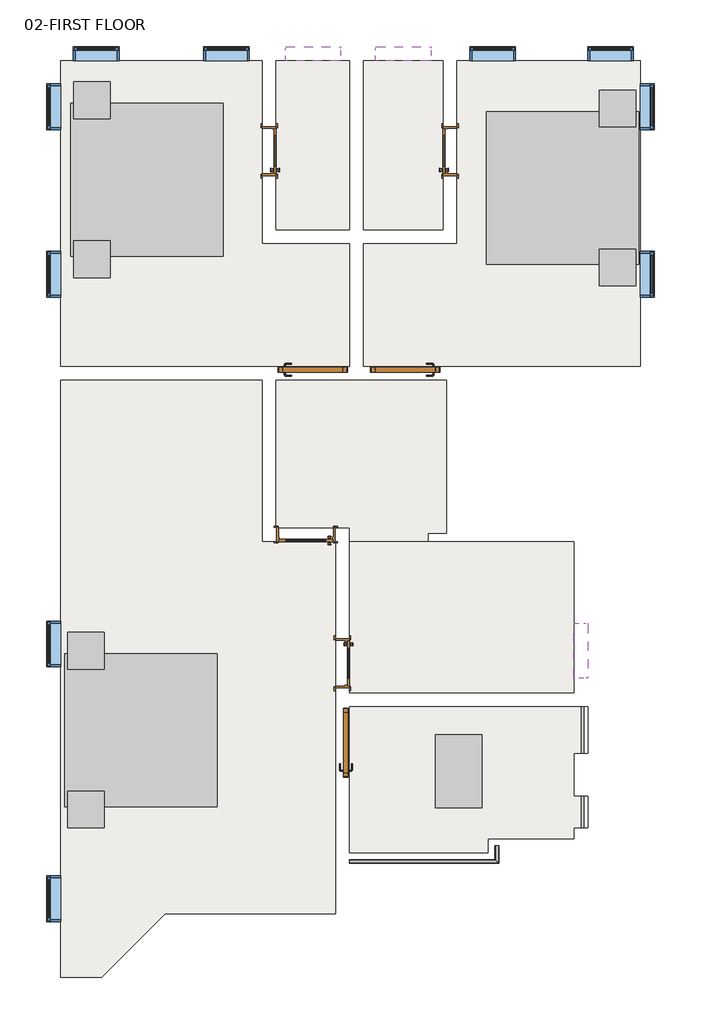
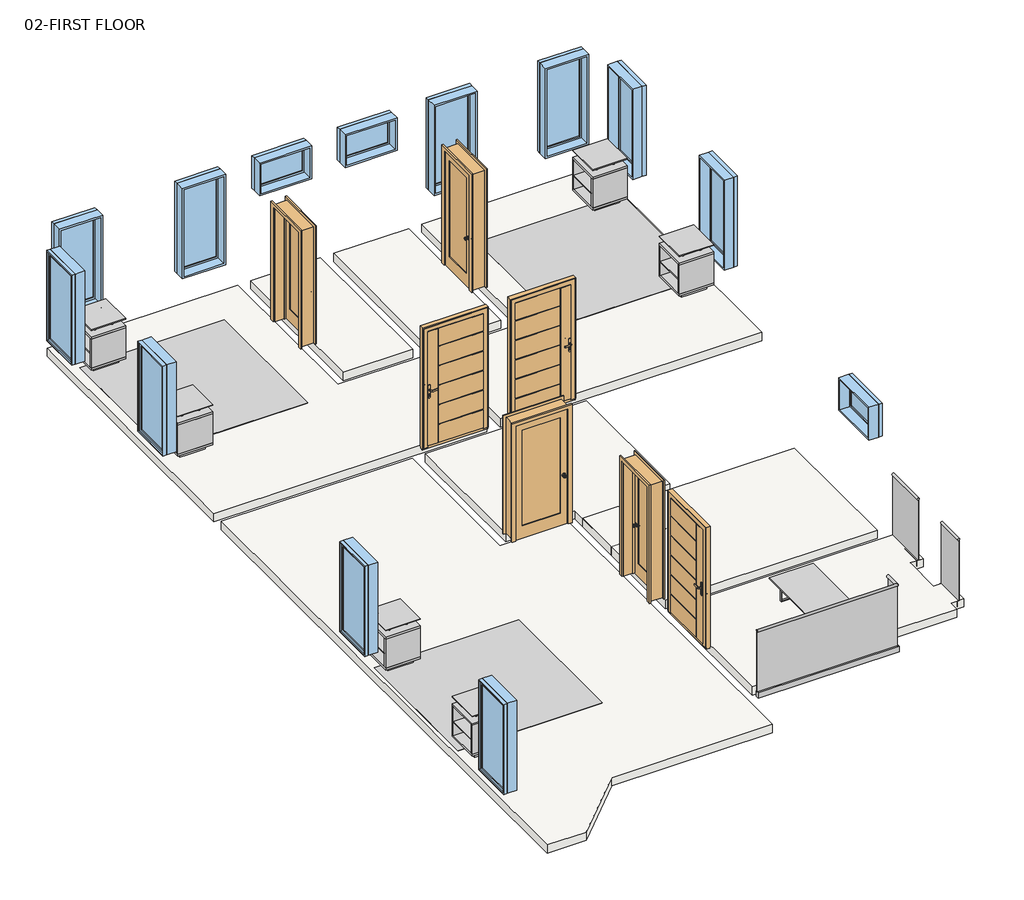
# One storey, incomplete: 13 windows, 10 furniture elements, 8 slabs, 7 doors, 3 railings.
"""IFC4 building model written with IfcOpenShell, lengths in millimetres."""

from ifc_helpers import new_model, si_unit, frame, origin, place, context, project, spatial, polyline, outline, extrude, transform, mapped, element, save
from components import door_1104_x_2190_mm_4e9de5db, door_1104_x_2190_mm_38c8fb91, m_door_interior_single_1_panel_wood_1ba8bb0f, m_door_interior_single_1_panel_wood_d9b71ff8, m_door_interior_single_1_panel_wood_d38da9c5, furniture_e65422ec, bed_table_10474_bed_table_10474_77ad9a9a, bed_table_10474_bed_table_10474_76a96b03, table_coffee_3_1200_x_760mm_bccf866f, railing_84ac703c, railing_926c3c2b, railing_f1bd4664, m_fixed_w2_a119b0d1, m_fixed_w4_tl_2657e552

model = new_model("IFC4")

# Units and contexts
model_context = context("Model", 3, world=origin())
ifc_project = project(units=[si_unit("LENGTHUNIT", "METRE", prefix="MILLI")], contexts=[model_context])

# Site, building, storey
site = spatial("IfcSite", under=ifc_project)
building = spatial("IfcBuilding", under=site)
storey = spatial("IfcBuildingStorey", under=building, Name="02-FIRST FLOOR", Elevation=3900.0)

# Doors
placement = place(None, origin())
door_1104_x_2190_mm_shape = door_1104_x_2190_mm_4e9de5db(model_context)
element("IfcDoor", 1, ObjectType="1104 x 2190 mm", at=placement, inside=storey, context=model_context, shape_type="MappedRepresentation", body=[
    mapped(door_1104_x_2190_mm_shape, transform((-4433.8712297, -202.0014262, 3900.0), x_axis=(-1.0, 0.0, 0.0), y_axis=(0.0, -1.0, 0.0), z_axis=(0.0, 0.0, 1.0))),
])
element("IfcDoor", 2, ObjectType="1104 x 2190 mm", at=placement, inside=storey, context=model_context, shape_type="MappedRepresentation", body=[
    mapped(door_1104_x_2190_mm_shape, transform((-5463.8712297, -6247.0014262, 3900.0), x_axis=(0.0, 1.0, 0.0), y_axis=(-1.0, 0.0, 0.0), z_axis=(0.0, 0.0, 1.0))),
])
door_1104_x_2190_mm_2_shape = door_1104_x_2190_mm_38c8fb91(model_context)
element("IfcDoor", 3, ObjectType="1104 x 2190 mm", at=placement, inside=storey, context=model_context, shape_type="MappedRepresentation", body=[
    mapped(door_1104_x_2190_mm_2_shape, transform((-5948.8712297, -202.0014262, 3900.0), x_axis=(1.0, 0.0, 0.0), y_axis=(0.0, 1.0, 0.0), z_axis=(0.0, 0.0, 1.0))),
])
m_door_interior_single_1_panel_wood_shape = m_door_interior_single_1_panel_wood_1ba8bb0f(model_context)
element("IfcDoor", 4, ObjectType="M_Door-Interior-Single-1_Panel-Wood", at=placement, inside=storey, context=model_context, shape_type="MappedRepresentation", body=[
    mapped(m_door_interior_single_1_panel_wood_shape, transform((-6660.6962297, 3432.9985738, 3900.0), x_axis=(0.0, 1.0, 0.0), y_axis=(-1.0, 0.0, 0.0), z_axis=(0.0, 0.0, 1.0))),
])
m_door_interior_single_1_panel_wood_2_shape = m_door_interior_single_1_panel_wood_d9b71ff8(model_context)
element("IfcDoor", 5, ObjectType="M_Door-Interior-Single-1_Panel-Wood", at=placement, inside=storey, context=model_context, shape_type="MappedRepresentation", body=[
    mapped(m_door_interior_single_1_panel_wood_2_shape, transform((-5460.6962297, -4947.0014262, 3900.0), x_axis=(0.0, -1.0, 0.0), y_axis=(1.0, 0.0, 0.0), z_axis=(0.0, 0.0, 1.0))),
])
element("IfcDoor", 6, ObjectType="M_Door-Interior-Single-1_Panel-Wood", at=placement, inside=storey, context=model_context, shape_type="MappedRepresentation", body=[
    mapped(m_door_interior_single_1_panel_wood_2_shape, transform((-3707.0462297, 3432.9985738, 3900.0), x_axis=(0.0, 1.0, 0.0), y_axis=(-1.0, 0.0, 0.0), z_axis=(0.0, 0.0, 1.0))),
])
m_door_interior_single_1_panel_wood_3_shape = m_door_interior_single_1_panel_wood_d38da9c5(model_context)
element("IfcDoor", 7, ObjectType="M_Door-Interior-Single-1_Panel-Wood", at=placement, inside=storey, context=model_context, shape_type="MappedRepresentation", body=[
    mapped(m_door_interior_single_1_panel_wood_3_shape, transform((-6063.8712297, -2843.6076238, 3900.0), x_axis=(-1.0, 0.0, 0.0), y_axis=(0.0, -1.0, 0.0), z_axis=(0.0, 0.0, 1.0))),
])

# Furniture
furniture_shape = furniture_e65422ec(model_context)
element("IfcFurniture", 8, at=placement, inside=storey, context=model_context, shape_type="MappedRepresentation", body=[
    mapped(furniture_shape, transform((-8763.9404049, -6041.0594341, 3900.0), x_axis=(0.0, -1.0, 0.0), y_axis=(1.0, 0.0, 0.0), z_axis=(0.0, 0.0, 1.0))),
])
element("IfcFurniture", 9, at=placement, inside=storey, context=model_context, shape_type="MappedRepresentation", body=[
    mapped(furniture_shape, transform((-8663.9404049, 2963.8544733, 3900.0), x_axis=(0.0, -1.0, 0.0), y_axis=(1.0, 0.0, 0.0), z_axis=(0.0, 0.0, 1.0))),
])
element("IfcFurniture", 10, at=placement, inside=storey, context=model_context, shape_type="MappedRepresentation", body=[
    mapped(furniture_shape, transform((-1858.8712297, 2827.9549908, 3900.0), x_axis=(0.0, 1.0, 0.0), y_axis=(-1.0, 0.0, 0.0), z_axis=(0.0, 0.0, 1.0))),
])
bed_table_10474_bed_table_10474_shape = bed_table_10474_bed_table_10474_77ad9a9a(model_context)
element("IfcFurniture", 11, ObjectType="Bed_Table_10474 : Bed_Table_10474", at=placement, inside=storey, context=model_context, shape_type="MappedRepresentation", body=[
    mapped(bed_table_10474_bed_table_10474_shape, transform((-9663.9404049, -7341.0594341, 3900.0), x_axis=(0.0, 1.0, 0.0), y_axis=(-1.0, 0.0, 0.0), z_axis=(0.0, 0.0, 1.0))),
])
element("IfcFurniture", 12, ObjectType="Bed_Table_10474 : Bed_Table_10474", at=placement, inside=storey, context=model_context, shape_type="MappedRepresentation", body=[
    mapped(bed_table_10474_bed_table_10474_shape, transform((-9563.9404049, 1663.8544733, 3900.0), x_axis=(0.0, 1.0, 0.0), y_axis=(-1.0, 0.0, 0.0), z_axis=(0.0, 0.0, 1.0))),
])
element("IfcFurniture", 13, ObjectType="Bed_Table_10474 : Bed_Table_10474", at=placement, inside=storey, context=model_context, shape_type="MappedRepresentation", body=[
    mapped(bed_table_10474_bed_table_10474_shape, transform((-958.8712297, 4127.9549908, 3900.0), x_axis=(0.0, -1.0, 0.0), y_axis=(1.0, 0.0, 0.0), z_axis=(0.0, 0.0, 1.0))),
])
bed_table_10474_bed_table_10474_2_shape = bed_table_10474_bed_table_10474_76a96b03(model_context)
element("IfcFurniture", 14, ObjectType="Bed_Table_10474 : Bed_Table_10474", at=placement, inside=storey, context=model_context, shape_type="MappedRepresentation", body=[
    mapped(bed_table_10474_bed_table_10474_2_shape, transform((-9663.9404049, -4741.0594341, 3900.0), x_axis=(0.0, -1.0, 0.0), y_axis=(1.0, 0.0, 0.0), z_axis=(0.0, 0.0, 1.0))),
])
element("IfcFurniture", 15, ObjectType="Bed_Table_10474 : Bed_Table_10474", at=placement, inside=storey, context=model_context, shape_type="MappedRepresentation", body=[
    mapped(bed_table_10474_bed_table_10474_2_shape, transform((-9563.9404049, 4263.8544733, 3900.0), x_axis=(0.0, -1.0, 0.0), y_axis=(1.0, 0.0, 0.0), z_axis=(0.0, 0.0, 1.0))),
])
element("IfcFurniture", 16, ObjectType="Bed_Table_10474 : Bed_Table_10474", at=placement, inside=storey, context=model_context, shape_type="MappedRepresentation", body=[
    mapped(bed_table_10474_bed_table_10474_2_shape, transform((-958.8712297, 1527.9549908, 3900.0), x_axis=(0.0, 1.0, 0.0), y_axis=(-1.0, 0.0, 0.0), z_axis=(0.0, 0.0, 1.0))),
])
table_coffee_3_1200_x_760mm_shape = table_coffee_3_1200_x_760mm_bccf866f(model_context)
element("IfcFurniture", 17, ObjectType="Table - Coffee (3) : 1200 x 760mm", at=placement, inside=storey, context=model_context, shape_type="MappedRepresentation", body=[
    mapped(table_coffee_3_1200_x_760mm_shape, transform((-3927.8698395, -6109.6891495, 3900.0), x_axis=(0.0, -1.0, 0.0), y_axis=(1.0, 0.0, 0.0), z_axis=(0.0, 0.0, 1.0))),
])

# Railings
railing_shape = railing_84ac703c(model_context)
element("IfcRailing", 18, at=placement, inside=storey, context=model_context, shape_type="MappedRepresentation", body=[
    mapped(railing_shape, transform((0.0, 0.0, 0.0), x_axis=(1.0, 0.0, 0.0), y_axis=(0.0, 1.0, 0.0), z_axis=(0.0, 0.0, 1.0))),
])
railing_2_shape = railing_926c3c2b(model_context)
element("IfcRailing", 19, at=placement, inside=storey, context=model_context, shape_type="MappedRepresentation", body=[
    mapped(railing_2_shape, transform((0.0, 0.0, 0.0), x_axis=(1.0, 0.0, 0.0), y_axis=(0.0, 1.0, 0.0), z_axis=(0.0, 0.0, 1.0))),
])
railing_3_shape = railing_f1bd4664(model_context)
element("IfcRailing", 20, at=placement, inside=storey, context=model_context, shape_type="MappedRepresentation", body=[
    mapped(railing_3_shape, transform((0.0, 0.0, 0.0), x_axis=(1.0, 0.0, 0.0), y_axis=(0.0, 1.0, 0.0), z_axis=(0.0, 0.0, 1.0))),
])

# Slabs
element("IfcSlab", 21, ObjectType="150", at=placement, inside=storey, context=model_context, shape_type="SweptSolid", body=[
    extrude(outline(polyline([(-10078.8712297, -317.0014262), (-6778.8712297, -317.0014262), (-6778.8712297, -2955.4326238), (-5578.8712297, -2955.4326238), (-5578.8712297, -9047.0014262), (-8363.4139709, -9047.0014262), (-9403.4139709, -10087.0014262), (-10078.8712297, -10087.0014262), (-10078.8712297, -317.0014262)])), frame((0.0, 0.0, 3750.0), z_axis=(0.0, 0.0, 1.0), x_axis=(1.0, 0.0, 0.0)), (0.0, 0.0, 1.0), 150.0),
])
element("IfcSlab", 22, ObjectType="150", at=placement, inside=storey, context=model_context, shape_type="SweptSolid", body=[
    extrude(outline(polyline([(-6778.8712297, 4912.9985738), (-6778.8712297, 1912.9985738), (-5348.8712297, 1912.9985738), (-5348.8712297, -87.0014262), (-10078.8712297, -87.0014262), (-10078.8712297, 4912.9985738), (-6778.8712297, 4912.9985738)])), frame((0.0, 0.0, 3750.0), z_axis=(0.0, 0.0, 1.0), x_axis=(1.0, 0.0, 0.0)), (0.0, 0.0, 1.0), 150.0),
])
element("IfcSlab", 23, ObjectType="150", at=placement, inside=storey, context=model_context, shape_type="SweptSolid", body=[
    extrude(outline(polyline([(-5118.8712297, 1912.9985738), (-3588.8712297, 1912.9985738), (-3588.8712297, 4912.9985738), (-588.8712297, 4912.9985738), (-588.8712297, -87.0014262), (-5118.8712297, -87.0014262), (-5118.8712297, 1912.9985738)])), frame((0.0, 0.0, 3750.0), z_axis=(0.0, 0.0, 1.0), x_axis=(1.0, 0.0, 0.0)), (0.0, 0.0, 1.0), 150.0),
])
element("IfcSlab", 24, ObjectType="150", at=placement, inside=storey, context=model_context, shape_type="SweptSolid", body=[
    extrude(outline(polyline([(-5348.8712297, -3817.0014262), (-5348.8712297, -2725.4326238), (-6548.8712297, -2725.4326238), (-6548.8712297, -317.0014262), (-3763.8712297, -317.0014262), (-3763.8712297, -2822.4014262), (-4063.8712297, -2822.4014262), (-4063.8712297, -3817.0014262), (-5348.8712297, -3817.0014262)])), frame((0.0, 0.0, 3750.0), z_axis=(0.0, 0.0, 1.0), x_axis=(1.0, 0.0, 0.0)), (0.0, 0.0, 1.0), 150.0),
])
element("IfcSlab", 25, ObjectType="150", at=placement, inside=storey, context=model_context, shape_type="SweptSolid", body=[
    extrude(outline(polyline([(-1448.8712297, -5662.0014262), (-1448.8712297, -6422.0014262), (-1678.8712297, -6422.0014262), (-1678.8712297, -7122.0014262), (-1448.8712297, -7122.0014262), (-1448.8712297, -7637.0014262), (-1678.8712297, -7637.0014262), (-1678.8712297, -7817.0014262), (-3078.8712297, -7817.0014262), (-3078.8712297, -8047.0014262), (-5348.8712297, -8047.0014262), (-5348.8712297, -5662.0014262), (-1448.8712297, -5662.0014262)])), frame((0.0, 0.0, 3750.0), z_axis=(0.0, 0.0, 1.0), x_axis=(1.0, 0.0, 0.0)), (0.0, 0.0, 1.0), 150.0),
])
element("IfcSlab", 26, ObjectType="150", at=placement, inside=storey, context=model_context, shape_type="SweptSolid", body=[
    extrude(outline(polyline([(-1678.8712297, -2955.4326238), (-1678.8712297, -5432.0014262), (-5348.8712297, -5432.0014262), (-5348.8712297, -2955.4326238), (-1678.8712297, -2955.4326238)])), frame((0.0, 0.0, 3750.0), z_axis=(0.0, 0.0, 1.0), x_axis=(1.0, 0.0, 0.0)), (0.0, 0.0, 1.0), 150.0),
])
element("IfcSlab", 27, ObjectType="150", at=placement, inside=storey, context=model_context, shape_type="SweptSolid", body=[
    extrude(outline(polyline([(-5348.8712297, 4912.9985738), (-5348.8712297, 2142.9985738), (-6548.8712297, 2142.9985738), (-6548.8712297, 4912.9985738), (-5348.8712297, 4912.9985738)])), frame((0.0, 0.0, 3750.0), z_axis=(0.0, 0.0, 1.0), x_axis=(1.0, 0.0, 0.0)), (0.0, 0.0, 1.0), 150.0),
])
element("IfcSlab", 28, ObjectType="150", at=placement, inside=storey, context=model_context, shape_type="SweptSolid", body=[
    extrude(outline(polyline([(-3818.8712297, 4912.9985738), (-3818.8712297, 2142.9985738), (-5118.8712297, 2142.9985738), (-5118.8712297, 4912.9985738), (-3818.8712297, 4912.9985738)])), frame((0.0, 0.0, 3750.0), z_axis=(0.0, 0.0, 1.0), x_axis=(1.0, 0.0, 0.0)), (0.0, 0.0, 1.0), 150.0),
])

# Windows
m_fixed_w2_shape = m_fixed_w2_a119b0d1(model_context)
element("IfcWindow", 29, ObjectType="M_Fixed : W2", at=placement, inside=storey, context=model_context, shape_type="MappedRepresentation", body=[
    mapped(m_fixed_w2_shape, transform((-7363.8712297, 5014.9985738, 3900.0), x_axis=(1.0, 0.0, 0.0), y_axis=(0.0, 1.0, 0.0), z_axis=(0.0, 0.0, 1.0))),
])
element("IfcWindow", 30, ObjectType="M_Fixed : W2", at=placement, inside=storey, context=model_context, shape_type="MappedRepresentation", body=[
    mapped(m_fixed_w2_shape, transform((-9493.8712297, 5014.9985738, 3900.0), x_axis=(1.0, 0.0, 0.0), y_axis=(0.0, 1.0, 0.0), z_axis=(0.0, 0.0, 1.0))),
])
element("IfcWindow", 31, ObjectType="M_Fixed : W2", at=placement, inside=storey, context=model_context, shape_type="MappedRepresentation", body=[
    mapped(m_fixed_w2_shape, transform((-10180.8712297, 4157.9985738, 3900.0), x_axis=(0.0, 1.0, 0.0), y_axis=(-1.0, 0.0, 0.0), z_axis=(0.0, 0.0, 1.0))),
])
element("IfcWindow", 32, ObjectType="M_Fixed : W2", at=placement, inside=storey, context=model_context, shape_type="MappedRepresentation", body=[
    mapped(m_fixed_w2_shape, transform((-10180.8712297, 1417.9985738, 3900.0), x_axis=(0.0, 1.0, 0.0), y_axis=(-1.0, 0.0, 0.0), z_axis=(0.0, 0.0, 1.0))),
])
element("IfcWindow", 33, ObjectType="M_Fixed : W2", at=placement, inside=storey, context=model_context, shape_type="MappedRepresentation", body=[
    mapped(m_fixed_w2_shape, transform((-3003.8712297, 5014.9985738, 3900.0), x_axis=(1.0, 0.0, 0.0), y_axis=(0.0, 1.0, 0.0), z_axis=(0.0, 0.0, 1.0))),
])
element("IfcWindow", 34, ObjectType="M_Fixed : W2", at=placement, inside=storey, context=model_context, shape_type="MappedRepresentation", body=[
    mapped(m_fixed_w2_shape, transform((-1073.8712297, 5014.9985738, 3900.0), x_axis=(1.0, 0.0, 0.0), y_axis=(0.0, 1.0, 0.0), z_axis=(0.0, 0.0, 1.0))),
])
element("IfcWindow", 35, ObjectType="M_Fixed : W2", at=placement, inside=storey, context=model_context, shape_type="MappedRepresentation", body=[
    mapped(m_fixed_w2_shape, transform((-486.8712297, 4157.9985738, 3900.0), x_axis=(0.0, -1.0, 0.0), y_axis=(1.0, 0.0, 0.0), z_axis=(0.0, 0.0, 1.0))),
])
element("IfcWindow", 36, ObjectType="M_Fixed : W2", at=placement, inside=storey, context=model_context, shape_type="MappedRepresentation", body=[
    mapped(m_fixed_w2_shape, transform((-486.8712297, 1417.9985738, 3900.0), x_axis=(0.0, -1.0, 0.0), y_axis=(1.0, 0.0, 0.0), z_axis=(0.0, 0.0, 1.0))),
])
element("IfcWindow", 37, ObjectType="M_Fixed : W2", at=placement, inside=storey, context=model_context, shape_type="MappedRepresentation", body=[
    mapped(m_fixed_w2_shape, transform((-10180.8712297, -4632.0014262, 3900.0), x_axis=(0.0, 1.0, 0.0), y_axis=(-1.0, 0.0, 0.0), z_axis=(0.0, 0.0, 1.0))),
])
element("IfcWindow", 38, ObjectType="M_Fixed : W2", at=placement, inside=storey, context=model_context, shape_type="MappedRepresentation", body=[
    mapped(m_fixed_w2_shape, transform((-10180.8712297, -8802.0014262, 3900.0), x_axis=(0.0, 1.0, 0.0), y_axis=(-1.0, 0.0, 0.0), z_axis=(0.0, 0.0, 1.0))),
])
m_fixed_w4_tl_shape = m_fixed_w4_tl_2657e552(model_context)
element("IfcWindow", 39, ObjectType="M_Fixed : W4 TL", at=placement, inside=storey, context=model_context, shape_type="MappedRepresentation", body=[
    mapped(m_fixed_w4_tl_shape, transform((-1576.8712297, -4739.5014262, 3900.0), x_axis=(0.0, -1.0, 0.0), y_axis=(1.0, 0.0, 0.0), z_axis=(0.0, 0.0, 1.0))),
])
element("IfcWindow", 40, ObjectType="M_Fixed : W4 TL", at=placement, inside=storey, context=model_context, shape_type="MappedRepresentation", body=[
    mapped(m_fixed_w4_tl_shape, transform((-4468.8712297, 5014.9985738, 3900.0), x_axis=(1.0, 0.0, 0.0), y_axis=(0.0, 1.0, 0.0), z_axis=(0.0, 0.0, 1.0))),
])
element("IfcWindow", 41, ObjectType="M_Fixed : W4 TL", at=placement, inside=storey, context=model_context, shape_type="MappedRepresentation", body=[
    mapped(m_fixed_w4_tl_shape, transform((-5948.8712297, 5014.9985738, 3900.0), x_axis=(1.0, 0.0, 0.0), y_axis=(0.0, 1.0, 0.0), z_axis=(0.0, 0.0, 1.0))),
])

save(model, "model.ifc")

# Revit data of these elements
# Type "1104 x 2190 mm"
#   Type Mark = "28"
#   Water resistance = "up to Class E900, EN 12208:2001"
#   Uniclass2015Version = "v1.21"
#   Uniclass2015Reference = "Ss_25_30_20_30"
#   Uniclass2015Description = "Frame and door leaf system"
#   URL = "www.aluprof.eu"
#   Type IFC Predefined Type = "USERDEFINED"
#   Right-hand / Left-hand door [instance default] = ""
#   Resistance to wind load = "up to Class C5/B5, EN 12210:2001"
#   Insert type = "ST"
#   Hardware [instance default] = ""
#   Product page = "https://aluprof.eu/en/architects/offer/window-and-door-systems/panel-doors#visualisation"
#   Operation = "SinglePanelOutwardOpening"
#   Opening type = "Outward"
#   NBSReference = "25-50-20/125"
#   NBSDescription = "Frame and door leaf system"
#   Important = "The actual acceptable construction dimensions are dependent on the selection of profiles and hardware, glazing type, construction weight and the construction’s operating conditions. These should be determined by a suitably qualified person, and using ALUPROF’s calculation software"
#   IfcExportType = "USERDEFINED"
#   IfcExportAs = "IfcDoorType"
#   Handle type [instance default] = ""
#   Manufacturer = "ALUPROF"
#   Export Type to IFC As = "IfcDoorType"
#   Door sill type [instance default] = ""
#   Description = "External single-leaf panel door outward opening"
#   Model = "MB-86 ST Panel Door AD07"
#   Content of the recyclate in the material = "69.2"
#   COBie.Type.WarrantyDurationParts = ""
#   COBie.Type.Name = ""
#   COBie.Type.Manufacturer = "ALUPROF S.A."
#   COBie.Space.Name = ""
#   COBie.Floor.Name = ""
#   COBie.Facility.Name = ""
#   COBie.CreatedOn = ""
#   COBie.Component.WarrantyStartDate = ""
#   COBie.Component.Name = "MB-86 ST Panel Door AD07"
#   Burglar resistance = "RC2"
#   Air permeability = "up to Class 4, EN 12207:2001"
#   Width of the active leaf = 1007.4 mm
#   Placement in wall = 20 mm
#   Thickness = 77 mm
#   Height of the opening sash = 2124.5 mm
#   Handle Offset = 1050 mm
#   Glazing thickness = 48 mm
#   Rough Height = 2250.7 mm
#   Rough Width = 1134.5 mm
#   Height = 2189.5 mm
#   Width = 1104.5 mm
#   Construction depth = 77 mm
#   Clear opening width = 900 mm
#   Clear opening height = 2100 mm
#   Height of the array = 341.583 mm
#   Schedule No. [instance default] = 1
#   Handrail = no
#   IsExternal = yes
#   Handle = yes
#   Door closer [instance default] = no
#   Function = 1
#   COBie.Type = yes
#   COBie = yes
#   Access control [instance default] = no
#   Panel = element 260956
#   Wall Closure = (empty or 0)
# Type "M_Door-Interior-Single-1_Panel-Wood"
#   Type Mark = "23"
#   Assembly Code = "C1020300"
#   Analytic Construction = "Wooden"
#   Top Rail = 120 mm
#   Thickness = 35 mm
#   Thermal Resistance (R) = 0.455703 (m²·K)/W
#   Swing Angle [instance default] = 90.00°
#   Stiles = 120 mm
#   Rough Width = 800 mm
#   Rough Height = 2125 mm
#   Height = 2100 mm
#   Width = 750 mm
#   Heat Transfer Coefficient (U) = 2.19465 W/(m²·K)
#   Bottom Rail = 230 mm
#   Trim Material = Cherry
#   Panel Material = Cherry
#   Frame Material = Cherry
#   Door Handle Material = Aluminum
#   Visual Light Transmittance = 0
#   Solar Heat Gain Coefficient = 0
#   Wall Closure = (empty or 0)
#   Function = (empty or 0)
# Type "M_Door-Interior-Single-1_Panel-Wood"
#   Type Mark = "26"
#   Assembly Code = "C1020300"
#   Analytic Construction = "Wooden"
#   Top Rail = 120 mm
#   Thickness = 35 mm
#   Thermal Resistance (R) = 0.455703 (m²·K)/W
#   Swing Angle [instance default] = 90.00°
#   Stiles = 120 mm
#   Rough Width = 950 mm
#   Rough Height = 2125 mm
#   Height = 2100 mm
#   Width = 900 mm
#   Heat Transfer Coefficient (U) = 2.19465 W/(m²·K)
#   Bottom Rail = 230 mm
#   Trim Material = Cherry
#   Panel Material = Cherry
#   Frame Material = Cherry
#   Door Handle Material = Aluminum
#   Visual Light Transmittance = 0
#   Solar Heat Gain Coefficient = 0
#   Wall Closure = (empty or 0)
#   Function = (empty or 0)
# Type
#   Width - Anchura = 2500 mm
#   Thickness - Espesor = 10 mm
#   Large - Largo = 2500 mm
#   Default Elevation = 1219.2 mm
# Type "Bed_Table_10474 : Bed_Table_10474"
#   myf = ""
#   Default Elevation = 0
# Type "Table - Coffee (3) : 1200 x 760mm"
#   Keynote = "N"
#   Height = 330 mm
#   Length = 1200 mm
#   Width = 760 mm
#   Material Base = Metal - Chrome
#   Material Top = Glass - Clear, Grey
#   Default Elevation = 0
#   Assembly Code = ""
# Type
#   Model = "Steel Pro handrail sidebased-LK60/Oak 40/12mm Glass"
#   Manufacturer = "Steelpro"
#   URL = "http://steelpro.bimobject.com/steelpro_lk"
#   Assembly Code = ""
#   built-in parameter 1008619 = -0.082021 (stored number, unit not read)
#   built-in parameter 1008612 = 0.0416667 (stored number, unit not read)
#   built-in parameter 1008611 = 0.0833333 (stored number, unit not read)
#   built-in parameter 1008609 = 4 (stored number, unit not read)
#   built-in parameter 1008604 = 0.166667 (stored number, unit not read)
#   built-in parameter 1008603 = 0.166667 (stored number, unit not read)
#   Railing Height = 1098 mm
#   built-in parameter 1008630 = 2
#   built-in parameter 1008610 = 1
#   built-in parameter 1008605 = 1
# Type "150"
#   Function = 0
#   Layers, outside or top first: 150 mm "J FLOOR" (function 1)
# Type "M_Fixed : W2"
#   Type Mark = "20"
#   Height = 1650 mm
#   Default Sill Height = 450 mm
#   Width = 750 mm
#   Window Inset = 19 mm
#   Frame Exterior Material = Iron, Ductile
#   Frame Interior Material = Iron, Ductile
#   Glass Pane Material = Glass
#   Sash = Iron, Ductile
#   Wall Closure = (empty or 0)
# Type "M_Fixed : W4 TL"
#   Type Mark = "22"
#   Height = 600 mm
#   Default Sill Height = 1500 mm
#   Width = 900 mm
#   Window Inset = 19 mm
#   Frame Exterior Material = Iron, Ductile
#   Frame Interior Material = Iron, Ductile
#   Glass Pane Material = Glass
#   Sash = Iron, Ductile
#   Wall Closure = (empty or 0)
# Elements 1, 2, 3 (IfcDoor, "1104 x 2190 mm")
#   Right-hand / Left-hand door = ""
#   Hardware = ""
#   Handle type = ""
#   Door sill type = ""
#   Schedule No. = 1
#   Door closer = no
#   Access control = no
#   Phase Created = New Construction
# Elements 4, 5, 6, 7 (IfcDoor, "M_Door-Interior-Single-1_Panel-Wood")
#   Swing Angle = 90.00°
#   Phase Created = New Construction
#   Materials on its faces: "Cherry", "Aluminum"
# Elements 8, 9, 10 (IfcFurniture)
#   Phase Created = New Construction
# Elements 11, 12, 13, 14, 15, 16 (IfcFurniture, "Bed_Table_10474 : Bed_Table_10474")
#   Phase Created = New Construction
#   Materials on its faces: "metal table", "madera", "glass table"
# Element 17 (IfcFurniture, "Table - Coffee (3) : 1200 x 760mm")
#   Phase Created = New Construction
#   Materials on its faces: "Metal - Chrome", "Glass - Clear, Grey"
# Elements 18, 19, 20 (IfcRailing)
#   Phase Created = New Construction
#   Materials on its faces: "Metal - Aluminum"
# Element 21 (IfcSlab, "150")
#   built-in parameter 1001955 = 1.5708 (stored number, unit not read)
#   Height Offset From Level = 0 mm
#   Phase Created = New Construction
#   Materials on its faces: "J FLOOR", "Wood 06, Chevron"
# Element 22 (IfcSlab, "150")
#   Height Offset From Level = 0 mm
#   Phase Created = New Construction
#   Materials on its faces: "J FLOOR", "Wood 04, Brick Bond"
# Element 23 (IfcSlab, "150")
#   built-in parameter 1001955 = 1.5708 (stored number, unit not read)
#   Height Offset From Level = 0 mm
#   Phase Created = New Construction
#   Materials on its faces: "J FLOOR", "Wood 04, Brick Bond"
# Element 24 (IfcSlab, "150")
#   built-in parameter 1001955 = 3.14159 (stored number, unit not read)
#   Height Offset From Level = 0 mm
#   Phase Created = New Construction
#   Materials on its faces: "J FLOOR", "Marble 05"
# Element 25 (IfcSlab, "150")
#   Height Offset From Level = 0 mm
#   Phase Created = New Construction
#   Materials on its faces: "J FLOOR", "Marble 05"
# Elements 26, 27, 28 (IfcSlab, "150")
#   Height Offset From Level = 0 mm
#   Phase Created = New Construction
#   Materials on its faces: "J FLOOR", "Tiles 13"
# Element 29 (IfcWindow, "M_Fixed : W2")
#   Mark = "19"
#   Phase Created = New Construction
#   Materials on its faces: "Iron, Ductile", "Glass"
# Element 30 (IfcWindow, "M_Fixed : W2")
#   Mark = "20"
#   Phase Created = New Construction
#   Materials on its faces: "Iron, Ductile", "Glass"
# Element 31 (IfcWindow, "M_Fixed : W2")
#   Mark = "21"
#   Phase Created = New Construction
#   Materials on its faces: "Iron, Ductile", "Glass"
# Element 32 (IfcWindow, "M_Fixed : W2")
#   Mark = "22"
#   Phase Created = New Construction
#   Materials on its faces: "Iron, Ductile", "Glass"
# Element 33 (IfcWindow, "M_Fixed : W2")
#   Mark = "23"
#   Phase Created = New Construction
#   Materials on its faces: "Iron, Ductile", "Glass"
# Element 34 (IfcWindow, "M_Fixed : W2")
#   Mark = "24"
#   Phase Created = New Construction
#   Materials on its faces: "Iron, Ductile", "Glass"
# Element 35 (IfcWindow, "M_Fixed : W2")
#   Mark = "25"
#   Phase Created = New Construction
#   Materials on its faces: "Iron, Ductile", "Glass"
# Element 36 (IfcWindow, "M_Fixed : W2")
#   Mark = "26"
#   Phase Created = New Construction
#   Materials on its faces: "Iron, Ductile", "Glass"
# Element 37 (IfcWindow, "M_Fixed : W2")
#   Mark = "27"
#   Phase Created = New Construction
#   Materials on its faces: "Iron, Ductile", "Glass"
# Element 38 (IfcWindow, "M_Fixed : W2")
#   Mark = "28"
#   Phase Created = New Construction
#   Materials on its faces: "Iron, Ductile", "Glass"
# Element 39 (IfcWindow, "M_Fixed : W4 TL")
#   Mark = "29"
#   Phase Created = New Construction
#   Materials on its faces: "Iron, Ductile", "Glass"
# Element 40 (IfcWindow, "M_Fixed : W4 TL")
#   Mark = "30"
#   Phase Created = New Construction
#   Materials on its faces: "Iron, Ductile", "Glass"
# Element 41 (IfcWindow, "M_Fixed : W4 TL")
#   Mark = "31"
#   Phase Created = New Construction
#   Materials on its faces: "Iron, Ductile", "Glass"
# Materials
#   "Cherry": class "Wood", colour RGB 154 107 61, transparency 0, Description = "Prunus Serotina", Cost = 0
#   "Aluminum": class "Metal", colour RGB 244 244 244, transparency 0, Description = "Aluminum 6061", Cost = 0
#   "Metal - Chrome": colour RGB 17 17 17, transparency 0
#   "Glass - Clear, Grey": colour RGB 252 255 255, transparency 0.64
#   "J FLOOR": class "Generic", colour RGB 255 255 255, transparency 0, Cost = 0
#   "Iron, Ductile": class "Metal", colour RGB 90 97 102, transparency 0, Description = "Ductile cast iron", Cost = 0
#   "Glass": class "Glass", colour RGB 218 227 224, transparency 0.85, Description = "Soda Lime Glass", Cost = 0
#   "metal table": class "Metal", colour RGB 168 168 168, transparency 0
#   "madera": class "Wood", colour RGB 191 159 105, transparency 0
#   "glass table": class "Glass", colour RGB 229 191 0, transparency 0.95
#   "Metal - Aluminum": colour RGB 247 247 247, transparency 0, Cost = 0
#   "Wood 06, Chevron": colour RGB 80 80 80, transparency 0
#   "Wood 04, Brick Bond": colour RGB 80 80 80, transparency 0
#   "Marble 05": colour RGB 80 80 80, transparency 0
#   "Tiles 13": colour RGB 80 80 80, transparency 0
# Room at (-4070.024, -4809.03) mm, phase "New Construction", upper level "02-FIRST FLOOR", upper offset 4000 mm, lower offset 0 mm
#   Number = "6"
# Room at (-4784.984, 3355.361) mm, phase "New Construction", upper level "02-FIRST FLOOR", upper offset 4000 mm, lower offset 0 mm
#   Number = "7"
# Room at (-5845.851, 3355.361) mm, phase "New Construction", upper level "02-FIRST FLOOR", upper offset 4000 mm, lower offset 0 mm
#   Number = "8"
# Room at (-8612.987, 2710.505) mm, phase "New Construction", upper level "02-FIRST FLOOR", upper offset 4000 mm, lower offset 0 mm
#   Number = "9"
#   Name = "Bedroom 2"
# Room at (-2489.867, 2520.505) mm, phase "New Construction", upper level "02-FIRST FLOOR", upper offset 4000 mm, lower offset 0 mm
#   Number = "10"
#   Name = "Bedroom 3"
# Room at (-7813.72, -6797.015) mm, phase "New Construction", upper level "02-FIRST FLOOR", upper offset 4000 mm, lower offset 0 mm
#   Number = "11"
#   Name = "Master Bedroom"
# Room at (-8382.515, -1456.771) mm, phase "New Construction", upper level "02-FIRST FLOOR", upper offset 4000 mm, lower offset 0 mm
#   Number = "12"
#   Name = "Room"
# Room at (-4008.758, -7020.41) mm, phase "New Construction", upper level "02-FIRST FLOOR", upper offset 4000 mm, lower offset 0 mm
#   Number = "13"
#   Name = "Balcony"
# Room at (-4947.024, -1185.506) mm, phase "New Construction", upper level "02-FIRST FLOOR", upper offset 4000 mm, lower offset 0 mm
#   Number = "14"
#   Name = "Room"
